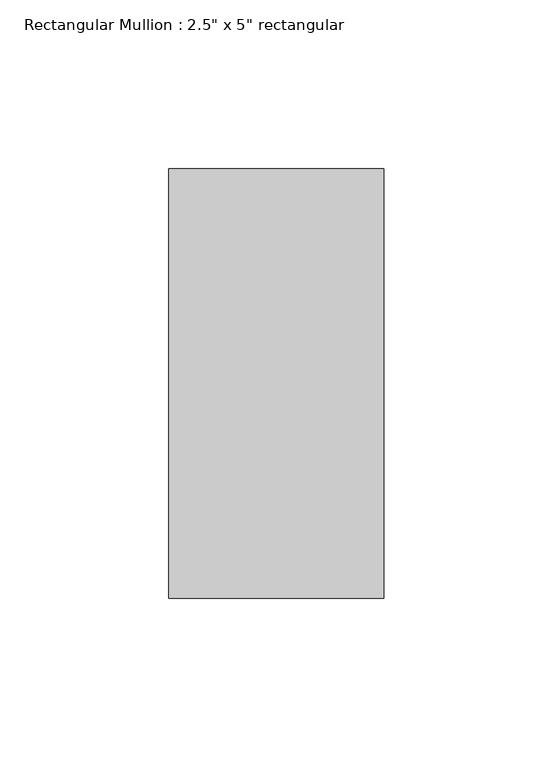
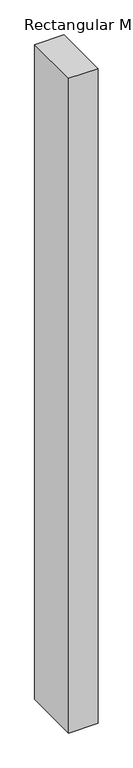
"""IFC4 building model written with IfcOpenShell, lengths in millimetres: member geometry."""

from ifc_helpers import new_model, si_unit, frame, origin, place, context, project, spatial, polyline, outline, extrude, source, transform, mapped, element, save


def member_56906109(model_context):
    return source(origin(), model_context, "Body", "SweptSolid", [
        extrude(outline(polyline([(31.75, 63.5), (31.75, -63.5), (-31.75, -63.5), (-31.75, 63.5), (31.75, 63.5)])), frame((0.0, 0.0, -1494.7499719), z_axis=(0.0, 0.0, 1.0), x_axis=(1.0, 0.0, 0.0)), (0.0, 0.0, 1.0), 1494.7499719),
    ])


if __name__ == "__main__":
    model = new_model("IFC4")
    model_context = context("Model", 3, world=origin())
    ifc_project = project(units=[si_unit("LENGTHUNIT", "METRE", prefix="MILLI")], contexts=[model_context])
    site = spatial("IfcSite", under=ifc_project)
    building = spatial("IfcBuilding", under=site)
    placement = place(None, origin())
    member_shape = member_56906109(model_context)
    element("IfcMember", 1, ObjectType="Rectangular Mullion : 2.5\" x 5\" rectangular", at=placement, inside=building, context=model_context, shape_type="MappedRepresentation", body=[
        mapped(member_shape, transform((0.0, 0.0, 0.0), x_axis=(1.0, 0.0, 0.0), y_axis=(0.0, 1.0, 0.0), z_axis=(0.0, 0.0, 1.0))),
    ])
    save(model, "model.ifc")

# Revit data of these elements
# Type "Rectangular Mullion : 2.5\" x 5\" rectangular"
#   built-in parameter 1007304 = 0.416667 (stored number, unit not read)
#   built-in parameter 1007301 = 0.104167 (stored number, unit not read)
#   built-in parameter 1007300 = 0.104167 (stored number, unit not read)
# Element 1 (IfcMember, "Rectangular Mullion : 2.5\" x 5\" rectangular")
#   Materials on its faces: "Aluminum"
# Materials
#   "Aluminum": class "Metal", colour RGB 247 247 247, transparency 0, Description = "Aluminum 6061", Cost = 0
